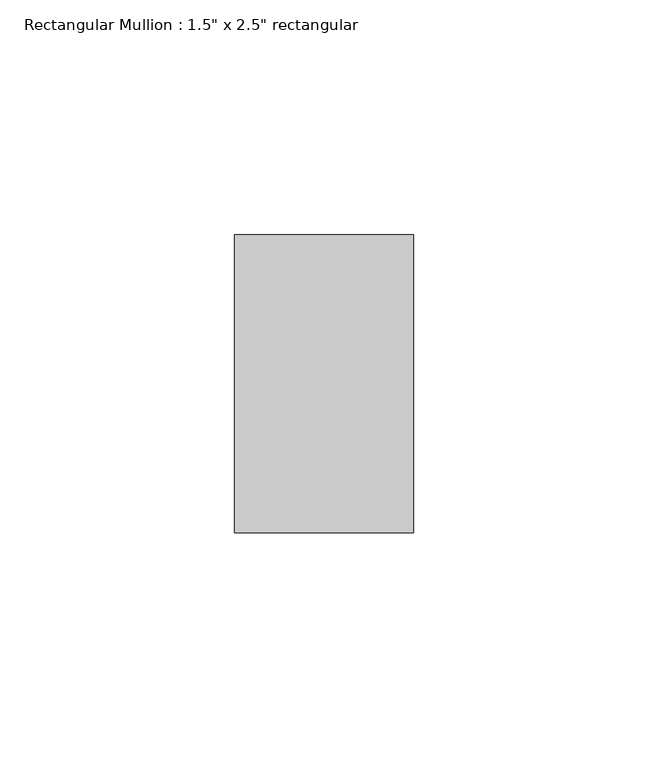
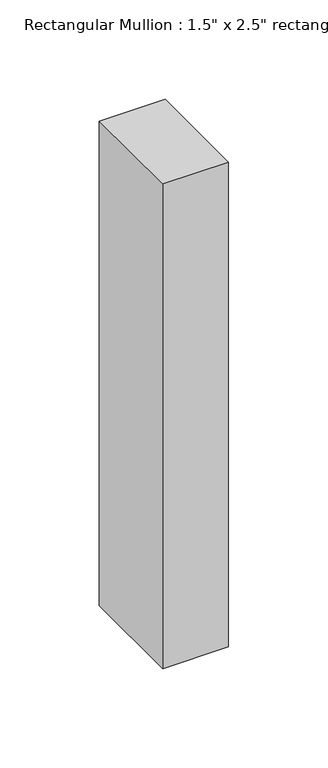
"""IFC4 building model written with IfcOpenShell, lengths in millimetres: member geometry."""

from ifc_helpers import new_model, si_unit, frame, origin, place, context, project, spatial, polyline, outline, extrude, source, transform, mapped, element, save


def member_b22cb31b(model_context):
    return source(origin(), model_context, "Body", "SweptSolid", [
        extrude(outline(polyline([(0.0, 31.75), (0.0, -31.75), (-38.1, -31.75), (-38.1, 31.75), (0.0, 31.75)])), frame((0.0, 0.0, -297.5334785), z_axis=(0.0, 0.0, 1.0), x_axis=(1.0, 0.0, 0.0)), (0.0, 0.0, 1.0), 297.5334785),
    ])


if __name__ == "__main__":
    model = new_model("IFC4")
    model_context = context("Model", 3, world=origin())
    ifc_project = project(units=[si_unit("LENGTHUNIT", "METRE", prefix="MILLI")], contexts=[model_context])
    site = spatial("IfcSite", under=ifc_project)
    building = spatial("IfcBuilding", under=site)
    placement = place(None, origin())
    member_shape = member_b22cb31b(model_context)
    element("IfcMember", 1, ObjectType="Rectangular Mullion : 1.5\" x 2.5\" rectangular", at=placement, inside=building, context=model_context, shape_type="MappedRepresentation", body=[
        mapped(member_shape, transform((0.0, 0.0, 0.0), x_axis=(1.0, 0.0, 0.0), y_axis=(0.0, 1.0, 0.0), z_axis=(0.0, 0.0, 1.0))),
    ])
    save(model, "model.ifc")

# Revit data of these elements
# Type "Rectangular Mullion : 1.5\" x 2.5\" rectangular"
#   built-in parameter 1007304 = 0.208333 (stored number, unit not read)
#   built-in parameter 1007301 = 0.0625 (stored number, unit not read)
#   built-in parameter 1007300 = 0.0625 (stored number, unit not read)
